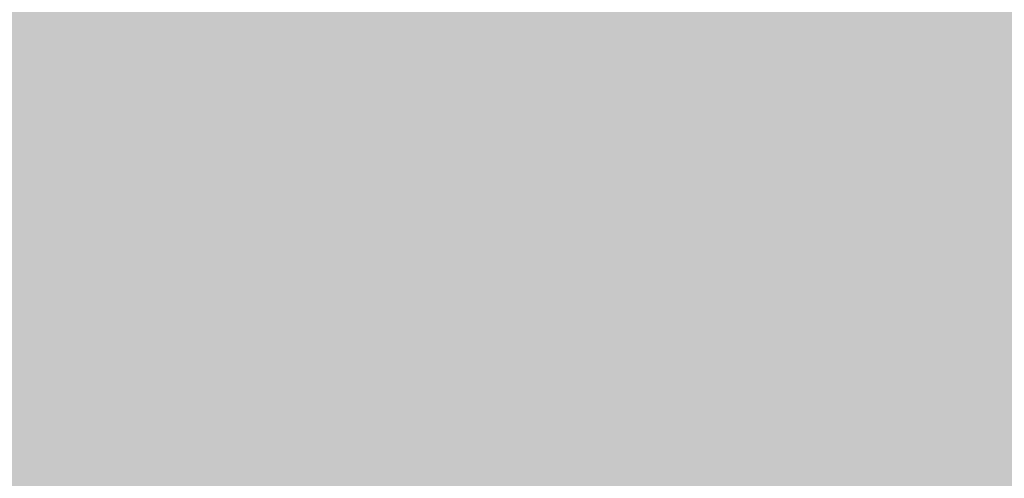
# Model space of a CAD drawing. Units: millimetres. Extents: x 0 to 2267, y 0 to 1823.
# Tile 176 of 256: x 1833.606 to 1838.83, y 1129.713 to 1132.147. Entities that reach past the tile are written whole.
import ezdxf

# ---------------------------------------------------------------- set-up
doc = ezdxf.new("R2010")
doc.units = ezdxf.units.MM
doc.header["$MEASUREMENT"] = 0
doc.layers.add('M-HATC', color=252, linetype='Continuous', lineweight=18)

msp = doc.modelspace()

# ---------------------------------------------------------------- hatches: boundary and pattern name
at = {"layer": 'M-HATC'}
h = msp.add_hatch(color=256, dxfattribs=at)
h.dxf.hatch_style = 1
h.paths.add_polyline_path([(2055.771, 1603.062), (1381.0868, 1603.062), (1381.0868, 1598.062), (2055.771, 1598.062)])
h.paths.add_polyline_path([(2055.771, 1598.062), (1381.0868, 1598.062), (1381.0868, 1593.062), (2055.771, 1593.062)])
h.paths.add_polyline_path([(2051.3074, 1536.7609), (1385.5504, 1536.7609), (1385.5504, 1526.7609), (1387.5504, 1526.7609), (1388.5366, 1525.0528), (1385.3319, 1521.2335), (1385.3319, 1521.2226), (2050.2542, 1522.7491), (2048.3212, 1525.0528), (2049.3074, 1526.7609), (2051.3074, 1526.7609)])
edge = h.paths.add_edge_path()
edge.add_arc((1847.5345, 1379.1492), 135, 222.603061, 222.890851, ccw=False)
edge.add_line((1748.1663, 1287.7656), (1683.0921, 1287.7656))
edge.add_arc((1583.7239, 1379.1492), 135, 317.109149, 317.396939, ccw=False)
edge.add_arc((1678.9686, 1290.6707), 5, 222.8909, 317.1091, ccw=False)
edge.add_arc((1774.2133, 1379.1492), 135, 222.603061, 222.890851, ccw=False)
edge.add_line((1674.8451, 1287.7656), (1609.7709, 1287.7656))
edge.add_arc((1510.4027, 1379.1492), 135, 317.109149, 317.396939, ccw=False)
edge.add_arc((1605.6474, 1290.6707), 5, 222.8909, 317.1091, ccw=False)
edge.add_arc((1700.8921, 1379.1492), 135, 222.603061, 222.890851, ccw=False)
edge.add_line((1601.5239, 1287.7656), (1536.4497, 1287.7656))
edge.add_arc((1437.0815, 1379.1492), 135, 317.109149, 317.396939, ccw=False)
edge.add_arc((1532.3262, 1290.6707), 5, 222.8909, 317.1091, ccw=False)
edge.add_arc((1627.5709, 1379.1492), 135, 222.603061, 222.890851, ccw=False)
edge.add_line((1528.2027, 1287.7656), (1505.9289, 1287.7656))
edge.add_spline(control_points=[(1505.9289, 1287.7656), (1504.2622, 1287.7656), (1504.2622, 1282.7656), (1505.9289, 1282.7656)], knot_values=[0, 0, 0, 0, 5, 5, 5, 5], degree=3, periodic=0)
edge.add_line((1505.9289, 1282.7656), (1930.9289, 1282.7656))
edge.add_spline(control_points=[(1930.9289, 1282.7656), (1932.5956, 1282.7656), (1932.5956, 1287.7656), (1930.9289, 1287.7656)], knot_values=[0, 0, 0, 0, 5, 5, 5, 5], degree=3, periodic=0)
edge.add_line((1930.9289, 1287.7656), (1903.0557, 1287.7656))
edge.add_arc((1803.6875, 1379.1492), 135, 317.109149, 317.396939, ccw=False)
edge.add_arc((1898.9322, 1290.6707), 5, 222.8909, 317.1091, ccw=False)
edge.add_arc((1994.1769, 1379.1492), 135, 222.603061, 222.890851, ccw=False)
edge.add_line((1894.8087, 1287.7656), (1829.7345, 1287.7656))
edge.add_arc((1730.3663, 1379.1492), 135, 317.109149, 317.396939, ccw=False)
edge.add_arc((1825.611, 1290.6707), 5, 222.8909, 317.1091, ccw=False)
edge.add_arc((1920.8557, 1379.1492), 135, 222.603061, 222.890851, ccw=False)
edge.add_line((1821.4875, 1287.7656), (1756.4133, 1287.7656))
edge.add_arc((1657.0451, 1379.1492), 135, 317.109149, 317.396939, ccw=False)
edge.add_arc((1752.2898, 1290.6707), 5, 222.8909, 317.1091, ccw=False)
edge = h.paths.add_edge_path()
edge.add_spline(control_points=[(1843.4289, 1227.2475), (1845.0956, 1227.2475), (1845.0956, 1232.2475), (1843.4289, 1232.2475)], knot_values=[0, 0, 0, 0, 5, 5, 5, 5], degree=3, periodic=0)
edge.add_line((1843.4289, 1232.2475), (1593.4289, 1232.2475))
edge.add_spline(control_points=[(1593.4289, 1232.2475), (1591.7622, 1232.2475), (1591.7622, 1227.2475), (1593.4289, 1227.2475)], knot_values=[0, 0, 0, 0, 5, 5, 5, 5], degree=3, periodic=0)
edge.add_line((1593.4289, 1227.2475), (1843.4289, 1227.2475))
h.paths.add_polyline_path([(1905.9289, 1127.4171), (1530.9289, 1127.4171, 0.414214), (1520.9289, 1117.4171), (1530.9289, 1117.4171), (1915.9289, 1117.4171, 0.414214)])
edge = h.paths.add_edge_path()
edge.add_arc((1397.0858, 1498.4078), 12.7299, 90.78215, 190.87871, ccw=False)
edge.add_line((1396.912, 1511.1365), (1428.0097, 1511.3488))
edge.add_line((1428.0097, 1511.3488), (1433.0097, 1511.3488))
edge.add_line((1433.0097, 1511.3488), (1434.439, 1511.3488))
edge.add_arc((1419.474, 1498.0804), 20, 41.561, 74.08211)
edge.add_line((1424.9592, 1517.3135), (1399.9351, 1517.2561))
edge.add_spline(control_points=[(1399.9307, 1517.2561), (1399.884, 1517.2131), (1399.8328, 1517.1689), (1399.7774, 1517.1236)], knot_values=[11.567499, 11.567499, 11.567499, 11.567499, 11.814249, 11.814249, 11.814249, 11.814249], degree=3, periodic=0)
edge.add_spline(control_points=[(1399.6328, 1517.0099), (1399.5831, 1516.9721), (1399.5307, 1516.9338), (1399.4759, 1516.8947)], knot_values=[11.167718, 11.167718, 11.167718, 11.167718, 11.365188, 11.365188, 11.365188, 11.365188], degree=3, periodic=0)
edge.add_spline(control_points=[(1399.3398, 1516.8001), (1399.1514, 1516.6719), (1398.9384, 1516.5377), (1398.704, 1516.3994)], knot_values=[10.376405, 10.376405, 10.376405, 10.376405, 11.00994, 11.00994, 11.00994, 11.00994], degree=3, periodic=0)
edge.add_spline(control_points=[(1398.6572, 1516.3719), (1398.5789, 1516.326), (1398.4983, 1516.2797), (1398.4155, 1516.2331)], knot_values=[10.125175, 10.125175, 10.125175, 10.125175, 10.334406, 10.334406, 10.334406, 10.334406], degree=3, periodic=0)
edge.add_spline(control_points=[(1398.2642, 1516.1487), (1398.196, 1516.1111), (1398.1263, 1516.0732), (1398.0555, 1516.0351)], knot_values=[9.832246, 9.832246, 9.832246, 9.832246, 9.999658, 9.999658, 9.999658, 9.999658], degree=3, periodic=0)
edge.add_spline(control_points=[(1397.9987, 1516.0048), (1397.7312, 1515.8621), (1397.446, 1515.7171), (1397.1466, 1515.5714)], knot_values=[9.161808, 9.161808, 9.161808, 9.161808, 9.787769, 9.787769, 9.787769, 9.787769], degree=3, periodic=0)
edge.add_spline(control_points=[(1397.1466, 1515.5714), (1396.8418, 1515.423), (1396.5222, 1515.274), (1396.1914, 1515.1262)], knot_values=[8.524455, 8.524455, 8.524455, 8.524455, 9.161808, 9.161808, 9.161808, 9.161808], degree=3, periodic=0)
edge.add_spline(control_points=[(1396.0777, 1515.0756), (1395.9854, 1515.0348), (1395.8922, 1514.994), (1395.7983, 1514.9534)], knot_values=[8.275193, 8.275193, 8.275193, 8.275193, 8.451726, 8.451726, 8.451726, 8.451726], degree=3, periodic=0)
edge.add_spline(control_points=[(1395.6018, 1514.8691), (1395.4997, 1514.8257), (1395.3968, 1514.7824), (1395.2932, 1514.7394)], knot_values=[7.962917, 7.962917, 7.962917, 7.962917, 8.152764, 8.152764, 8.152764, 8.152764], degree=3, periodic=0)
edge.add_spline(control_points=[(1395.2116, 1514.7057), (1394.8278, 1514.5475), (1394.4345, 1514.3929), (1394.0364, 1514.2442)], knot_values=[7.21254, 7.21254, 7.21254, 7.21254, 7.913148, 7.913148, 7.913148, 7.913148], degree=3, periodic=0)
edge.add_spline(control_points=[(1394.0364, 1514.2442), (1393.7076, 1514.1214), (1393.3754, 1514.0027), (1393.0427, 1513.8895)], knot_values=[6.633733, 6.633733, 6.633733, 6.633733, 7.21254, 7.21254, 7.21254, 7.21254], degree=3, periodic=0)
edge.add_spline(control_points=[(1392.8214, 1513.815), (1392.7198, 1513.7812), (1392.6181, 1513.7479), (1392.5166, 1513.7152)], knot_values=[6.328796, 6.328796, 6.328796, 6.328796, 6.505493, 6.505493, 6.505493, 6.505493], degree=3, periodic=0)
edge.add_spline(control_points=[(1392.5166, 1513.7152), (1392.3187, 1513.6515), (1392.1212, 1513.59), (1391.9244, 1513.531)], knot_values=[5.984605, 5.984605, 5.984605, 5.984605, 6.328796, 6.328796, 6.328796, 6.328796], degree=3, periodic=0)
edge.add_spline(control_points=[(1391.7915, 1513.4915), (1391.3122, 1513.3501), (1390.8384, 1513.2239), (1390.3784, 1513.1171)], knot_values=[5.066697, 5.066697, 5.066697, 5.066697, 5.907055, 5.907055, 5.907055, 5.907055], degree=3, periodic=0)
edge.add_spline(control_points=[(1390.3784, 1513.1171), (1390.1797, 1513.071), (1389.9836, 1513.0284), (1389.7907, 1512.9899)], knot_values=[4.70367, 4.70367, 4.70367, 4.70367, 5.066695, 5.066695, 5.066695, 5.066695], degree=3, periodic=0)
edge.add_spline(control_points=[(1389.422, 1512.9204), (1389.2459, 1512.8892), (1389.0729, 1512.8617), (1388.9036, 1512.8381)], knot_values=[4.130571, 4.130571, 4.130571, 4.130571, 4.469816, 4.469816, 4.469816, 4.469816], degree=3, periodic=0)
edge.add_spline(control_points=[(1388.9036, 1512.8381), (1388.591, 1512.7946), (1388.2911, 1512.7644), (1388.0071, 1512.7494)], knot_values=[3.504031, 3.504031, 3.504031, 3.504031, 4.130571, 4.130571, 4.130571, 4.130571], degree=3, periodic=0)
edge.add_spline(control_points=[(1387.9356, 1512.7459), (1387.8538, 1512.7423), (1387.7733, 1512.74), (1387.6944, 1512.739)], knot_values=[3.268866, 3.268866, 3.268866, 3.268866, 3.451164, 3.451164, 3.451164, 3.451164], degree=3, periodic=0)
edge.add_spline(control_points=[(1387.3351, 1512.7443), (1387.2076, 1512.7499), (1387.0847, 1512.7597), (1386.967, 1512.7739)], knot_values=[2.670686, 2.670686, 2.670686, 2.670686, 2.984, 2.984, 2.984, 2.984], degree=3, periodic=0)
edge.add_spline(control_points=[(1386.8327, 1512.7922), (1386.8209, 1512.7941), (1386.8092, 1512.7959), (1386.7975, 1512.7979)], knot_values=[2.516981, 2.516981, 2.516981, 2.516981, 2.549528, 2.549528, 2.549528, 2.549528], degree=3, periodic=0)
edge.add_spline(control_points=[(1386.4526, 1512.8735), (1386.4257, 1512.881), (1386.3993, 1512.889), (1386.3733, 1512.8972)], knot_values=[2.095869, 2.095869, 2.095869, 2.095869, 2.17941, 2.17941, 2.17941, 2.17941], degree=3, periodic=0)
edge.add_spline(control_points=[(1386.0691, 1513.0189), (1386.0634, 1513.0217), (1386.0577, 1513.0246), (1386.052, 1513.0275)], knot_values=[1.72453, 1.72453, 1.72453, 1.72453, 1.745933, 1.745933, 1.745933, 1.745933], degree=3, periodic=0)
edge.add_arc((1399.474, 1498.0804), 20, 131.82432, 180)
edge.add_arc((1630.3336, 1505.5484), 250.9708, 181.705176, 236.427975)
edge.add_arc((1605.3399, 1483.3044), 218.7822, 238.660829, 243.34961)
edge.add_arc((1647.0911, 1510.3592), 262.8986, 183.129836, 237.853442, ccw=False)
h.paths.add_polyline_path([(1406.5369, 1391.9644, 0.149382), (1491.5506, 1296.4418, -0.129517)], flags=17)
edge = h.paths.add_edge_path()
edge.add_arc((2037.3838, 1498.0804), 20, 0, 48.26587)
edge.add_spline(control_points=[(2050.6973, 1513.0052), (2050.6512, 1512.9847), (2050.6034, 1512.9655), (2050.5539, 1512.9477)], knot_values=[1.835652, 1.835652, 1.835652, 1.835652, 2.000781, 2.000781, 2.000781, 2.000781], degree=3, periodic=0)
edge.add_spline(control_points=[(2050.4616, 1512.9166), (2050.479, 1512.9221), (2050.4963, 1512.9277), (2050.5133, 1512.9335)], knot_values=[2.045477, 2.045477, 2.045477, 2.045477, 2.101389, 2.101389, 2.101389, 2.101389], degree=3, periodic=0)
edge.add_spline(control_points=[(2050.129, 1512.8342), (2050.1984, 1512.8473), (2050.2657, 1512.8623), (2050.3308, 1512.8792)], knot_values=[2.237629, 2.237629, 2.237629, 2.237629, 2.435841, 2.435841, 2.435841, 2.435841], degree=3, periodic=0)
edge.add_spline(control_points=[(2050.0946, 1512.8278), (2050.1061, 1512.8299), (2050.1176, 1512.832), (2050.129, 1512.8342)], knot_values=[2.435841, 2.435841, 2.435841, 2.435841, 2.468321, 2.468321, 2.468321, 2.468321], degree=3, periodic=0)
edge.add_spline(control_points=[(2049.7843, 1512.7851), (2049.8552, 1512.7922), (2049.9243, 1512.8008), (2049.9917, 1512.8109)], knot_values=[2.563852, 2.563852, 2.563852, 2.563852, 2.748541, 2.748541, 2.748541, 2.748541], degree=3, periodic=0)
edge.add_spline(control_points=[(2049.4052, 1512.7617), (2049.5364, 1512.7653), (2049.6629, 1512.773), (2049.7843, 1512.7851)], knot_values=[2.748541, 2.748541, 2.748541, 2.748541, 3.064882, 3.064882, 3.064882, 3.064882], degree=3, periodic=0)
edge.add_spline(control_points=[(2049.1698, 1512.7597), (2049.2336, 1512.7591), (2049.2965, 1512.7594), (2049.3584, 1512.7606)], knot_values=[3.102309, 3.102309, 3.102309, 3.102309, 3.2503, 3.2503, 3.2503, 3.2503], degree=3, periodic=0)
edge.add_spline(control_points=[(2048.8573, 1512.7691), (2048.9638, 1512.7638), (2049.068, 1512.7606), (2049.1698, 1512.7597)], knot_values=[3.2503, 3.2503, 3.2503, 3.2503, 3.486069, 3.486069, 3.486069, 3.486069], degree=3, periodic=0)
edge.add_spline(control_points=[(2048.6924, 1512.7789), (2048.3729, 1512.8009), (2048.0345, 1512.8411), (2047.6817, 1512.897)], knot_values=[3.606429, 3.606429, 3.606429, 3.606429, 4.2989, 4.2989, 4.2989, 4.2989], degree=3, periodic=0)
edge.add_spline(control_points=[(2047.6817, 1512.897), (2047.5458, 1512.9185), (2047.4077, 1512.9424), (2047.2678, 1512.9685)], knot_values=[4.2989, 4.2989, 4.2989, 4.2989, 4.565769, 4.565769, 4.565769, 4.565769], degree=3, periodic=0)
edge.add_spline(control_points=[(2047.2678, 1512.9685), (2047.1449, 1512.9914), (2047.0207, 1513.016), (2046.8951, 1513.0422)], knot_values=[4.565769, 4.565769, 4.565769, 4.565769, 4.799971, 4.799971, 4.799971, 4.799971], degree=3, periodic=0)
edge.add_spline(control_points=[(2046.8951, 1513.0422), (2046.5286, 1513.1188), (2046.1513, 1513.209), (2045.7676, 1513.3107)], knot_values=[4.799971, 4.799971, 4.799971, 4.799971, 5.483718, 5.483718, 5.483718, 5.483718], degree=3, periodic=0)
edge.add_spline(control_points=[(2045.7676, 1513.3107), (2045.3724, 1513.4154), (2044.9704, 1513.5322), (2044.5662, 1513.6588)], knot_values=[5.483718, 5.483718, 5.483718, 5.483718, 6.187866, 6.187866, 6.187866, 6.187866], degree=3, periodic=0)
edge.add_spline(control_points=[(2044.5662, 1513.6588), (2044.4149, 1513.7061), (2044.2633, 1513.7549), (2044.1116, 1513.8048)], knot_values=[6.187866, 6.187866, 6.187866, 6.187866, 6.451551, 6.451551, 6.451551, 6.451551], degree=3, periodic=0)
edge.add_spline(control_points=[(2044.1116, 1513.8048), (2043.9967, 1513.8427), (2043.8817, 1513.8813), (2043.7668, 1513.9205)], knot_values=[6.451551, 6.451551, 6.451551, 6.451551, 6.651434, 6.651434, 6.651434, 6.651434], degree=3, periodic=0)
edge.add_spline(control_points=[(2043.7668, 1513.9205), (2043.3716, 1514.0554), (2042.9774, 1514.1979), (2042.5886, 1514.3458)], knot_values=[6.651434, 6.651434, 6.651434, 6.651434, 7.338879, 7.338879, 7.338879, 7.338879], degree=3, periodic=0)
edge.add_spline(control_points=[(2042.5886, 1514.3458), (2042.1643, 1514.5071), (2041.7465, 1514.6749), (2041.3409, 1514.846)], knot_values=[7.338879, 7.338879, 7.338879, 7.338879, 8.089209, 8.089209, 8.089209, 8.089209], degree=3, periodic=0)
edge.add_spline(control_points=[(2041.3409, 1514.846), (2041.1028, 1514.9465), (2040.869, 1515.0481), (2040.6405, 1515.1502)], knot_values=[8.089209, 8.089209, 8.089209, 8.089209, 8.529587, 8.529587, 8.529587, 8.529587], degree=3, periodic=0)
edge.add_spline(control_points=[(2040.51, 1515.2089), (2040.0824, 1515.4022), (2039.6747, 1515.5971), (2039.295, 1515.7894)], knot_values=[8.613818, 8.613818, 8.613818, 8.613818, 9.44571, 9.44571, 9.44571, 9.44571], degree=3, periodic=0)
edge.add_spline(control_points=[(2039.295, 1515.7894), (2039.0618, 1515.9075), (2038.8391, 1516.0246), (2038.6288, 1516.1398)], knot_values=[9.44571, 9.44571, 9.44571, 9.44571, 9.956404, 9.956404, 9.956404, 9.956404], degree=3, periodic=0)
edge.add_spline(control_points=[(2038.6288, 1516.1398), (2038.5187, 1516.2001), (2038.4121, 1516.2598), (2038.309, 1516.3189)], knot_values=[9.956404, 9.956404, 9.956404, 9.956404, 10.223542, 10.223542, 10.223542, 10.223542], degree=3, periodic=0)
edge.add_spline(control_points=[(2038.309, 1516.3189), (2038.2138, 1516.3735), (2038.1216, 1516.4276), (2038.0328, 1516.481)], knot_values=[10.223542, 10.223542, 10.223542, 10.223542, 10.47051, 10.47051, 10.47051, 10.47051], degree=3, periodic=0)
edge.add_spline(control_points=[(2038.0328, 1516.481), (2037.7855, 1516.6296), (2037.5639, 1516.773), (2037.3722, 1516.909)], knot_values=[10.47051, 10.47051, 10.47051, 10.47051, 11.15767, 11.15767, 11.15767, 11.15767], degree=3, periodic=0)
edge.add_spline(control_points=[(2037.3722, 1516.909), (2037.2789, 1516.9752), (2037.1927, 1517.0396), (2037.1142, 1517.102)], knot_values=[11.15767, 11.15767, 11.15767, 11.15767, 11.49227, 11.49227, 11.49227, 11.49227], degree=3, periodic=0)
edge.add_spline(control_points=[(2036.8564, 1517.3259), (2036.9148, 1517.2692), (2036.9814, 1517.2103), (2037.0557, 1517.1492)], knot_values=[11.577341, 11.577341, 11.577341, 11.577341, 11.91035, 11.91035, 11.91035, 11.91035], degree=3, periodic=0)
edge.add_spline(control_points=[(2036.8074, 1517.3748), (2036.823, 1517.3587), (2036.8393, 1517.3424), (2036.8564, 1517.3259)], knot_values=[11.91035, 11.91035, 11.91035, 11.91035, 12.007402, 12.007402, 12.007402, 12.007402], degree=3, periodic=0)
edge.add_spline(control_points=[(2036.7017, 1517.494), (2036.7104, 1517.483), (2036.7196, 1517.4719), (2036.7291, 1517.4606)], knot_values=[12.184155, 12.184155, 12.184155, 12.184155, 12.255409, 12.255409, 12.255409, 12.255409], degree=3, periodic=0)
edge.add_spline(control_points=[(2036.6159, 1517.6205), (2036.62, 1517.613), (2036.6243, 1517.6055), (2036.6289, 1517.5979)], knot_values=[12.487913, 12.487913, 12.487913, 12.487913, 12.541035, 12.541035, 12.541035, 12.541035], degree=3, periodic=0)
edge.add_spline(control_points=[(2036.5635, 1517.786), (2036.5637, 1517.7794), (2036.5642, 1517.7726), (2036.565, 1517.7658)], knot_values=[12.911761, 12.911761, 12.911761, 12.911761, 12.968286, 12.968286, 12.968286, 12.968286], degree=3, periodic=0)
edge.add_spline(control_points=[(2036.6166, 1517.9304), (2036.6125, 1517.9259), (2036.6086, 1517.9212), (2036.6049, 1517.9165)], knot_values=[13.382527, 13.382527, 13.382527, 13.382527, 13.433791, 13.433791, 13.433791, 13.433791], degree=3, periodic=0)
edge.add_spline(control_points=[(2036.749, 1518.017), (2036.7361, 1518.0116), (2036.7239, 1518.006), (2036.7124, 1518.0002)], knot_values=[13.726299, 13.726299, 13.726299, 13.726299, 13.809928, 13.809928, 13.809928, 13.809928], degree=3, periodic=0)
edge.add_spline(control_points=[(2036.8604, 1518.0528), (2036.8386, 1518.0474), (2036.8181, 1518.0416), (2036.7988, 1518.0353)], knot_values=[13.910887, 13.910887, 13.910887, 13.910887, 14.02153, 14.02153, 14.02153, 14.02153], degree=3, periodic=0)
edge.add_line((2036.9639, 1518.0804), (2032.3838, 1518.0804))
edge.add_line((2032.3838, 1518.0804), (2027.3838, 1518.0804))
edge.add_line((2027.3838, 1518.0804), (2022.3838, 1518.0804))
edge.add_line((2022.3838, 1518.0804), (2017.3838, 1518.0804))
edge.add_arc((2017.3838, 1498.0804), 20, 90, 138.439)
edge.add_line((2002.4188, 1511.3488), (2003.8481, 1511.3488))
edge.add_line((2003.8481, 1511.3488), (2008.8481, 1511.3488))
edge.add_line((2008.8481, 1511.3488), (2039.772, 1511.1377))
edge.add_arc((2039.772, 1498.4078), 12.7299, -10.87871, 90, ccw=False)
edge.add_arc((1789.7668, 1510.3592), 262.8986, 302.146558, 356.870164, ccw=False)
edge.add_arc((1831.5179, 1483.3044), 218.7822, 296.65039, 301.339171)
edge.add_arc((1806.5242, 1505.5484), 250.9708, 303.572025, 358.294824)
h.paths.add_polyline_path([(2030.321, 1391.9644, -0.129517), (1945.3072, 1296.4418, 0.149382)], flags=17)
edge = h.paths.add_edge_path()
edge.add_spline(control_points=[(2037.2464, 1518.0821), (2037.2898, 1518.081), (2037.3355, 1518.0804), (2037.3838, 1518.0804)], knot_values=[0.000012, 0.000012, 0.000012, 0.000012, 0.144754, 0.144754, 0.144754, 0.144754], degree=3, periodic=0)
edge.add_line((2037.3357, 1518.0804), (2037.0096, 1518.0804))
edge.add_spline(control_points=[(2037.0096, 1518.0804), (2036.9822, 1518.0768), (2036.956, 1518.0727), (2036.9312, 1518.0681)], knot_values=[14.13465, 14.13465, 14.13465, 14.13465, 14.247197, 14.247197, 14.247197, 14.247197], degree=3, periodic=0)
edge.add_spline(control_points=[(2036.9312, 1518.0681), (2036.9276, 1518.0674), (2036.9241, 1518.0667), (2036.9205, 1518.0661)], knot_values=[14.118315, 14.118315, 14.118315, 14.118315, 14.13465, 14.13465, 14.13465, 14.13465], degree=3, periodic=0)
edge.add_spline(control_points=[(2036.9205, 1518.0661), (2036.9118, 1518.0644), (2036.9032, 1518.0626), (2036.8948, 1518.0608)], knot_values=[14.078086, 14.078086, 14.078086, 14.078086, 14.118315, 14.118315, 14.118315, 14.118315], degree=3, periodic=0)
edge.add_spline(control_points=[(2036.8948, 1518.0608), (2036.883, 1518.0583), (2036.8716, 1518.0556), (2036.8604, 1518.0528)], knot_values=[14.02153, 14.02153, 14.02153, 14.02153, 14.078086, 14.078086, 14.078086, 14.078086], degree=3, periodic=0)
edge.add_spline(control_points=[(2036.8604, 1518.0528), (2036.8386, 1518.0474), (2036.8181, 1518.0416), (2036.7988, 1518.0353)], knot_values=[13.910887, 13.910887, 13.910887, 13.910887, 14.02153, 14.02153, 14.02153, 14.02153], degree=3, periodic=0)
edge.add_spline(control_points=[(2036.7988, 1518.0353), (2036.7981, 1518.035), (2036.7974, 1518.0348), (2036.7967, 1518.0346)], knot_values=[13.906906, 13.906906, 13.906906, 13.906906, 13.910887, 13.910887, 13.910887, 13.910887], degree=3, periodic=0)
edge.add_spline(control_points=[(2036.7967, 1518.0346), (2036.7882, 1518.0318), (2036.7799, 1518.0289), (2036.7719, 1518.0259)], knot_values=[13.857826, 13.857826, 13.857826, 13.857826, 13.906906, 13.906906, 13.906906, 13.906906], degree=3, periodic=0)
edge.add_spline(control_points=[(2036.7719, 1518.0259), (2036.764, 1518.023), (2036.7564, 1518.02), (2036.749, 1518.017)], knot_values=[13.809928, 13.809928, 13.809928, 13.809928, 13.857826, 13.857826, 13.857826, 13.857826], degree=3, periodic=0)
edge.add_spline(control_points=[(2036.749, 1518.017), (2036.7361, 1518.0116), (2036.7239, 1518.006), (2036.7124, 1518.0002)], knot_values=[13.726299, 13.726299, 13.726299, 13.726299, 13.809928, 13.809928, 13.809928, 13.809928], degree=3, periodic=0)
edge.add_spline(control_points=[(2036.7124, 1518.0002), (2036.7121, 1518), (2036.7118, 1517.9999), (2036.7115, 1517.9997)], knot_values=[13.723993, 13.723993, 13.723993, 13.723993, 13.726299, 13.726299, 13.726299, 13.726299], degree=3, periodic=0)
edge.add_spline(control_points=[(2036.7115, 1517.9997), (2036.7063, 1517.9971), (2036.7013, 1517.9944), (2036.6965, 1517.9917)], knot_values=[13.686536, 13.686536, 13.686536, 13.686536, 13.723993, 13.723993, 13.723993, 13.723993], degree=3, periodic=0)
edge.add_spline(control_points=[(2036.6965, 1517.9917), (2036.6919, 1517.9891), (2036.6874, 1517.9865), (2036.6831, 1517.9839)], knot_values=[13.651251, 13.651251, 13.651251, 13.651251, 13.686536, 13.686536, 13.686536, 13.686536], degree=3, periodic=0)
edge.add_spline(control_points=[(2036.6831, 1517.9839), (2036.6764, 1517.9798), (2036.67, 1517.9757), (2036.6639, 1517.9714)], knot_values=[13.596804, 13.596804, 13.596804, 13.596804, 13.651251, 13.651251, 13.651251, 13.651251], degree=3, periodic=0)
edge.add_spline(control_points=[(2036.6639, 1517.9714), (2036.6636, 1517.9712), (2036.6633, 1517.9709), (2036.6629, 1517.9707)], knot_values=[13.593956, 13.593956, 13.593956, 13.593956, 13.596804, 13.596804, 13.596804, 13.596804], degree=3, periodic=0)
edge.add_spline(control_points=[(2036.6629, 1517.9707), (2036.6603, 1517.9689), (2036.6577, 1517.967), (2036.6552, 1517.9651)], knot_values=[13.570322, 13.570322, 13.570322, 13.570322, 13.593956, 13.593956, 13.593956, 13.593956], degree=3, periodic=0)
edge.add_spline(control_points=[(2036.6552, 1517.9651), (2036.6525, 1517.9631), (2036.6499, 1517.9611), (2036.6474, 1517.9591)], knot_values=[13.545477, 13.545477, 13.545477, 13.545477, 13.570322, 13.570322, 13.570322, 13.570322], degree=3, periodic=0)
edge.add_spline(control_points=[(2036.6474, 1517.9591), (2036.6472, 1517.9589), (2036.6471, 1517.9588), (2036.6469, 1517.9587)], knot_values=[13.543931, 13.543931, 13.543931, 13.543931, 13.545477, 13.545477, 13.545477, 13.545477], degree=3, periodic=0)
edge.add_spline(control_points=[(2036.6469, 1517.9587), (2036.6412, 1517.9541), (2036.6358, 1517.9494), (2036.6307, 1517.9447)], knot_values=[13.488237, 13.488237, 13.488237, 13.488237, 13.543931, 13.543931, 13.543931, 13.543931], degree=3, periodic=0)
edge.add_spline(control_points=[(2036.6307, 1517.9447), (2036.6282, 1517.9423), (2036.6257, 1517.9399), (2036.6233, 1517.9374)], knot_values=[13.460307, 13.460307, 13.460307, 13.460307, 13.488237, 13.488237, 13.488237, 13.488237], degree=3, periodic=0)
edge.add_spline(control_points=[(2036.6233, 1517.9374), (2036.6215, 1517.9356), (2036.6198, 1517.9338), (2036.6181, 1517.932)], knot_values=[13.439712, 13.439712, 13.439712, 13.439712, 13.460307, 13.460307, 13.460307, 13.460307], degree=3, periodic=0)
edge.add_spline(control_points=[(2036.6181, 1517.932), (2036.6176, 1517.9315), (2036.6171, 1517.9309), (2036.6166, 1517.9304)], knot_values=[13.433791, 13.433791, 13.433791, 13.433791, 13.439712, 13.439712, 13.439712, 13.439712], degree=3, periodic=0)
edge.add_spline(control_points=[(2036.6166, 1517.9304), (2036.6125, 1517.9259), (2036.6086, 1517.9212), (2036.6049, 1517.9165)], knot_values=[13.382527, 13.382527, 13.382527, 13.382527, 13.433791, 13.433791, 13.433791, 13.433791], degree=3, periodic=0)
edge.add_spline(control_points=[(2036.6049, 1517.9165), (2036.6026, 1517.9135), (2036.6004, 1517.9104), (2036.5982, 1517.9074)], knot_values=[13.350017, 13.350017, 13.350017, 13.350017, 13.382527, 13.382527, 13.382527, 13.382527], degree=3, periodic=0)
edge.add_spline(control_points=[(2036.5982, 1517.9074), (2036.5972, 1517.9059), (2036.5962, 1517.9043), (2036.5952, 1517.9028)], knot_values=[13.333922, 13.333922, 13.333922, 13.333922, 13.350017, 13.350017, 13.350017, 13.350017], degree=3, periodic=0)
edge.add_spline(control_points=[(2036.5952, 1517.9028), (2036.5945, 1517.9018), (2036.5939, 1517.9009), (2036.5933, 1517.8999)], knot_values=[13.323828, 13.323828, 13.323828, 13.323828, 13.333922, 13.333922, 13.333922, 13.333922], degree=3, periodic=0)
edge.add_spline(control_points=[(2036.5933, 1517.8999), (2036.5905, 1517.8955), (2036.5879, 1517.8909), (2036.5855, 1517.8864)], knot_values=[13.277545, 13.277545, 13.277545, 13.277545, 13.323828, 13.323828, 13.323828, 13.323828], degree=3, periodic=0)
edge.add_spline(control_points=[(2036.5855, 1517.8864), (2036.5836, 1517.8827), (2036.5817, 1517.8789), (2036.5801, 1517.8751)], knot_values=[13.240119, 13.240119, 13.240119, 13.240119, 13.277545, 13.277545, 13.277545, 13.277545], degree=3, periodic=0)
edge.add_spline(control_points=[(2036.5801, 1517.8751), (2036.5795, 1517.8739), (2036.579, 1517.8727), (2036.5785, 1517.8715)], knot_values=[13.228211, 13.228211, 13.228211, 13.228211, 13.240119, 13.240119, 13.240119, 13.240119], degree=3, periodic=0)
edge.add_spline(control_points=[(2036.5785, 1517.8715), (2036.578, 1517.8702), (2036.5774, 1517.869), (2036.5769, 1517.8677)], knot_values=[13.215717, 13.215717, 13.215717, 13.215717, 13.228211, 13.228211, 13.228211, 13.228211], degree=3, periodic=0)
edge.add_spline(control_points=[(2036.5769, 1517.8677), (2036.5755, 1517.864), (2036.5741, 1517.8603), (2036.5729, 1517.8565)], knot_values=[13.179847, 13.179847, 13.179847, 13.179847, 13.215717, 13.215717, 13.215717, 13.215717], degree=3, periodic=0)
edge.add_spline(control_points=[(2036.5729, 1517.8565), (2036.5713, 1517.8515), (2036.5699, 1517.8464), (2036.5687, 1517.8413)], knot_values=[13.132017, 13.132017, 13.132017, 13.132017, 13.179847, 13.179847, 13.179847, 13.179847], degree=3, periodic=0)
edge.add_spline(control_points=[(2036.5687, 1517.8413), (2036.5684, 1517.8402), (2036.5682, 1517.8392), (2036.568, 1517.8382)], knot_values=[13.122482, 13.122482, 13.122482, 13.122482, 13.132017, 13.132017, 13.132017, 13.132017], degree=3, periodic=0)
edge.add_spline(control_points=[(2036.568, 1517.8382), (2036.5676, 1517.8363), (2036.5672, 1517.8345), (2036.5669, 1517.8327)], knot_values=[13.105592, 13.105592, 13.105592, 13.105592, 13.122482, 13.122482, 13.122482, 13.122482], degree=3, periodic=0)
edge.add_spline(control_points=[(2036.5669, 1517.8327), (2036.5662, 1517.8292), (2036.5657, 1517.8257), (2036.5652, 1517.8222)], knot_values=[13.074063, 13.074063, 13.074063, 13.074063, 13.105592, 13.105592, 13.105592, 13.105592], degree=3, periodic=0)
edge.add_spline(control_points=[(2036.5652, 1517.8222), (2036.5652, 1517.8222), (2036.5652, 1517.8222), (2036.5652, 1517.8222)], knot_values=[13.074043, 13.074043, 13.074043, 13.074043, 13.074063, 13.074063, 13.074063, 13.074063], degree=3, periodic=0)
edge.add_spline(control_points=[(2036.5652, 1517.8222), (2036.5644, 1517.8164), (2036.5639, 1517.8106), (2036.5636, 1517.8046)], knot_values=[13.021884, 13.021884, 13.021884, 13.021884, 13.074043, 13.074043, 13.074043, 13.074043], degree=3, periodic=0)
edge.add_spline(control_points=[(2036.5636, 1517.8046), (2036.5636, 1517.804), (2036.5636, 1517.8034), (2036.5635, 1517.8028)], knot_values=[13.01674, 13.01674, 13.01674, 13.01674, 13.021884, 13.021884, 13.021884, 13.021884], degree=3, periodic=0)
edge.add_spline(control_points=[(2036.5635, 1517.8028), (2036.5634, 1517.8005), (2036.5634, 1517.7982), (2036.5634, 1517.7958)], knot_values=[12.996438, 12.996438, 12.996438, 12.996438, 13.01674, 13.01674, 13.01674, 13.01674], degree=3, periodic=0)
edge.add_spline(control_points=[(2036.5634, 1517.7958), (2036.5633, 1517.7926), (2036.5634, 1517.7893), (2036.5635, 1517.786)], knot_values=[12.968286, 12.968286, 12.968286, 12.968286, 12.996438, 12.996438, 12.996438, 12.996438], degree=3, periodic=0)
edge.add_spline(control_points=[(2036.5635, 1517.786), (2036.5637, 1517.7794), (2036.5642, 1517.7726), (2036.565, 1517.7658)], knot_values=[12.911761, 12.911761, 12.911761, 12.911761, 12.968286, 12.968286, 12.968286, 12.968286], degree=3, periodic=0)
edge.add_spline(control_points=[(2036.565, 1517.7658), (2036.565, 1517.7657), (2036.565, 1517.7656), (2036.565, 1517.7656)], knot_values=[12.911017, 12.911017, 12.911017, 12.911017, 12.911761, 12.911761, 12.911761, 12.911761], degree=3, periodic=0)
edge.add_spline(control_points=[(2036.565, 1517.7656), (2036.5654, 1517.7625), (2036.5658, 1517.7593), (2036.5663, 1517.7562)], knot_values=[12.88528, 12.88528, 12.88528, 12.88528, 12.911017, 12.911017, 12.911017, 12.911017], degree=3, periodic=0)
edge.add_spline(control_points=[(2036.5663, 1517.7562), (2036.5667, 1517.7534), (2036.5672, 1517.7506), (2036.5677, 1517.7478)], knot_values=[12.862519, 12.862519, 12.862519, 12.862519, 12.88528, 12.88528, 12.88528, 12.88528], degree=3, periodic=0)
edge.add_spline(control_points=[(2036.5677, 1517.7478), (2036.5678, 1517.7474), (2036.5679, 1517.7469), (2036.568, 1517.7465)], knot_values=[12.858885, 12.858885, 12.858885, 12.858885, 12.862519, 12.862519, 12.862519, 12.862519], degree=3, periodic=0)
edge.add_spline(control_points=[(2036.568, 1517.7465), (2036.5692, 1517.7399), (2036.5707, 1517.7332), (2036.5724, 1517.7264)], knot_values=[12.8053, 12.8053, 12.8053, 12.8053, 12.858885, 12.858885, 12.858885, 12.858885], degree=3, periodic=0)
edge.add_spline(control_points=[(2036.5724, 1517.7264), (2036.5734, 1517.7226), (2036.5745, 1517.7187), (2036.5756, 1517.7149)], knot_values=[12.775176, 12.775176, 12.775176, 12.775176, 12.8053, 12.8053, 12.8053, 12.8053], degree=3, periodic=0)
edge.add_spline(control_points=[(2036.5756, 1517.7149), (2036.5763, 1517.7125), (2036.577, 1517.7102), (2036.5778, 1517.7078)], knot_values=[12.756759, 12.756759, 12.756759, 12.756759, 12.775176, 12.775176, 12.775176, 12.775176], degree=3, periodic=0)
edge.add_spline(control_points=[(2036.5778, 1517.7078), (2036.5781, 1517.7067), (2036.5784, 1517.7057), (2036.5787, 1517.7047)], knot_values=[12.748742, 12.748742, 12.748742, 12.748742, 12.756759, 12.756759, 12.756759, 12.756759], degree=3, periodic=0)
edge.add_spline(control_points=[(2036.5787, 1517.7047), (2036.5808, 1517.6983), (2036.5831, 1517.6919), (2036.5856, 1517.6854)], knot_values=[12.69959, 12.69959, 12.69959, 12.69959, 12.748742, 12.748742, 12.748742, 12.748742], degree=3, periodic=0)
edge.add_spline(control_points=[(2036.5856, 1517.6854), (2036.5876, 1517.68), (2036.5898, 1517.6746), (2036.5921, 1517.6692)], knot_values=[12.659038, 12.659038, 12.659038, 12.659038, 12.69959, 12.69959, 12.69959, 12.69959], degree=3, periodic=0)
edge.add_spline(control_points=[(2036.5921, 1517.6692), (2036.594, 1517.6648), (2036.5959, 1517.6605), (2036.5979, 1517.6561)], knot_values=[12.626806, 12.626806, 12.626806, 12.626806, 12.659038, 12.659038, 12.659038, 12.659038], degree=3, periodic=0)
edge.add_spline(control_points=[(2036.5979, 1517.6561), (2036.5984, 1517.6551), (2036.5989, 1517.6541), (2036.5993, 1517.6531)], knot_values=[12.619394, 12.619394, 12.619394, 12.619394, 12.626806, 12.626806, 12.626806, 12.626806], degree=3, periodic=0)
edge.add_spline(control_points=[(2036.5993, 1517.6531), (2036.6043, 1517.6424), (2036.6099, 1517.6315), (2036.6159, 1517.6205)], knot_values=[12.541039, 12.541039, 12.541039, 12.541039, 12.619394, 12.619394, 12.619394, 12.619394], degree=3, periodic=0)
edge.add_spline(control_points=[(2036.6159, 1517.6205), (2036.6159, 1517.6205), (2036.6159, 1517.6205), (2036.6159, 1517.6205)], knot_values=[12.541035, 12.541035, 12.541035, 12.541035, 12.541039, 12.541039, 12.541039, 12.541039], degree=3, periodic=0)
edge.add_spline(control_points=[(2036.6159, 1517.6205), (2036.62, 1517.613), (2036.6243, 1517.6055), (2036.6289, 1517.5979)], knot_values=[12.487913, 12.487913, 12.487913, 12.487913, 12.541035, 12.541035, 12.541035, 12.541035], degree=3, periodic=0)
edge.add_spline(control_points=[(2036.6289, 1517.5979), (2036.6326, 1517.5916), (2036.6365, 1517.5853), (2036.6406, 1517.5789)], knot_values=[12.443982, 12.443982, 12.443982, 12.443982, 12.487913, 12.487913, 12.487913, 12.487913], degree=3, periodic=0)
edge.add_spline(control_points=[(2036.6406, 1517.5789), (2036.6414, 1517.5776), (2036.6423, 1517.5763), (2036.6431, 1517.5749)], knot_values=[12.434996, 12.434996, 12.434996, 12.434996, 12.443982, 12.443982, 12.443982, 12.443982], degree=3, periodic=0)
edge.add_spline(control_points=[(2036.6431, 1517.5749), (2036.6531, 1517.5596), (2036.6639, 1517.5439), (2036.6756, 1517.528)], knot_values=[12.329647, 12.329647, 12.329647, 12.329647, 12.434996, 12.434996, 12.434996, 12.434996], degree=3, periodic=0)
edge.add_spline(control_points=[(2036.6756, 1517.528), (2036.6839, 1517.5168), (2036.6925, 1517.5055), (2036.7017, 1517.494)], knot_values=[12.255409, 12.255409, 12.255409, 12.255409, 12.329647, 12.329647, 12.329647, 12.329647], degree=3, periodic=0)
edge.add_spline(control_points=[(2036.7017, 1517.494), (2036.7104, 1517.483), (2036.7196, 1517.4719), (2036.7291, 1517.4606)], knot_values=[12.184155, 12.184155, 12.184155, 12.184155, 12.255409, 12.255409, 12.255409, 12.255409], degree=3, periodic=0)
edge.add_spline(control_points=[(2036.7291, 1517.4606), (2036.7436, 1517.4435), (2036.759, 1517.4262), (2036.7753, 1517.4085)], knot_values=[12.075961, 12.075961, 12.075961, 12.075961, 12.184155, 12.184155, 12.184155, 12.184155], degree=3, periodic=0)
edge.add_spline(control_points=[(2036.7753, 1517.4085), (2036.7763, 1517.4075), (2036.7773, 1517.4064), (2036.7783, 1517.4054)], knot_values=[12.069502, 12.069502, 12.069502, 12.069502, 12.075961, 12.075961, 12.075961, 12.075961], degree=3, periodic=0)
edge.add_spline(control_points=[(2036.7783, 1517.4054), (2036.7877, 1517.3953), (2036.7974, 1517.385), (2036.8074, 1517.3748)], knot_values=[12.007402, 12.007402, 12.007402, 12.007402, 12.069502, 12.069502, 12.069502, 12.069502], degree=3, periodic=0)
edge.add_spline(control_points=[(2036.8074, 1517.3748), (2036.823, 1517.3587), (2036.8393, 1517.3424), (2036.8564, 1517.3259)], knot_values=[11.91035, 11.91035, 11.91035, 11.91035, 12.007402, 12.007402, 12.007402, 12.007402], degree=3, periodic=0)
edge.add_spline(control_points=[(2036.8564, 1517.3259), (2036.9148, 1517.2692), (2036.9814, 1517.2103), (2037.0557, 1517.1492)], knot_values=[11.577341, 11.577341, 11.577341, 11.577341, 11.91035, 11.91035, 11.91035, 11.91035], degree=3, periodic=0)
edge.add_spline(control_points=[(2037.0557, 1517.1492), (2037.0747, 1517.1336), (2037.0942, 1517.1179), (2037.1142, 1517.102)], knot_values=[11.49227, 11.49227, 11.49227, 11.49227, 11.577341, 11.577341, 11.577341, 11.577341], degree=3, periodic=0)
edge.add_spline(control_points=[(2037.1142, 1517.102), (2037.1927, 1517.0396), (2037.2789, 1516.9752), (2037.3722, 1516.909)], knot_values=[11.15767, 11.15767, 11.15767, 11.15767, 11.49227, 11.49227, 11.49227, 11.49227], degree=3, periodic=0)
edge.add_spline(control_points=[(2037.3722, 1516.909), (2037.5639, 1516.773), (2037.7855, 1516.6296), (2038.0328, 1516.481)], knot_values=[10.47051, 10.47051, 10.47051, 10.47051, 11.15767, 11.15767, 11.15767, 11.15767], degree=3, periodic=0)
edge.add_spline(control_points=[(2038.0328, 1516.481), (2038.1216, 1516.4276), (2038.2138, 1516.3735), (2038.309, 1516.3189)], knot_values=[10.223542, 10.223542, 10.223542, 10.223542, 10.47051, 10.47051, 10.47051, 10.47051], degree=3, periodic=0)
edge.add_spline(control_points=[(2038.309, 1516.3189), (2038.4121, 1516.2598), (2038.5187, 1516.2001), (2038.6288, 1516.1398)], knot_values=[9.956404, 9.956404, 9.956404, 9.956404, 10.223542, 10.223542, 10.223542, 10.223542], degree=3, periodic=0)
edge.add_spline(control_points=[(2038.6288, 1516.1398), (2038.8391, 1516.0246), (2039.0618, 1515.9075), (2039.295, 1515.7894)], knot_values=[9.44571, 9.44571, 9.44571, 9.44571, 9.956404, 9.956404, 9.956404, 9.956404], degree=3, periodic=0)
edge.add_spline(control_points=[(2039.295, 1515.7894), (2039.6747, 1515.5971), (2040.0824, 1515.4022), (2040.51, 1515.2089)], knot_values=[8.613818, 8.613818, 8.613818, 8.613818, 9.44571, 9.44571, 9.44571, 9.44571], degree=3, periodic=0)
edge.add_spline(control_points=[(2040.51, 1515.2089), (2040.5533, 1515.1893), (2040.5968, 1515.1697), (2040.6405, 1515.1502)], knot_values=[8.529587, 8.529587, 8.529587, 8.529587, 8.613818, 8.613818, 8.613818, 8.613818], degree=3, periodic=0)
edge.add_spline(control_points=[(2040.6405, 1515.1502), (2040.869, 1515.0481), (2041.1028, 1514.9465), (2041.3409, 1514.846)], knot_values=[8.089209, 8.089209, 8.089209, 8.089209, 8.529587, 8.529587, 8.529587, 8.529587], degree=3, periodic=0)
edge.add_spline(control_points=[(2041.3409, 1514.846), (2041.7465, 1514.6749), (2042.1643, 1514.5071), (2042.5886, 1514.3458)], knot_values=[7.338879, 7.338879, 7.338879, 7.338879, 8.089209, 8.089209, 8.089209, 8.089209], degree=3, periodic=0)
edge.add_spline(control_points=[(2042.5886, 1514.3458), (2042.9774, 1514.1979), (2043.3716, 1514.0554), (2043.7668, 1513.9205)], knot_values=[6.651434, 6.651434, 6.651434, 6.651434, 7.338879, 7.338879, 7.338879, 7.338879], degree=3, periodic=0)
edge.add_spline(control_points=[(2043.7668, 1513.9205), (2043.8817, 1513.8813), (2043.9967, 1513.8427), (2044.1116, 1513.8048)], knot_values=[6.451551, 6.451551, 6.451551, 6.451551, 6.651434, 6.651434, 6.651434, 6.651434], degree=3, periodic=0)
edge.add_spline(control_points=[(2044.1116, 1513.8048), (2044.2633, 1513.7549), (2044.4149, 1513.7061), (2044.5662, 1513.6588)], knot_values=[6.187866, 6.187866, 6.187866, 6.187866, 6.451551, 6.451551, 6.451551, 6.451551], degree=3, periodic=0)
edge.add_spline(control_points=[(2044.5662, 1513.6588), (2044.9704, 1513.5322), (2045.3724, 1513.4154), (2045.7676, 1513.3107)], knot_values=[5.483718, 5.483718, 5.483718, 5.483718, 6.187866, 6.187866, 6.187866, 6.187866], degree=3, periodic=0)
edge.add_spline(control_points=[(2045.7676, 1513.3107), (2046.1513, 1513.209), (2046.5286, 1513.1188), (2046.8951, 1513.0422)], knot_values=[4.799971, 4.799971, 4.799971, 4.799971, 5.483718, 5.483718, 5.483718, 5.483718], degree=3, periodic=0)
edge.add_spline(control_points=[(2046.8951, 1513.0422), (2047.0207, 1513.016), (2047.1449, 1512.9914), (2047.2678, 1512.9685)], knot_values=[4.565769, 4.565769, 4.565769, 4.565769, 4.799971, 4.799971, 4.799971, 4.799971], degree=3, periodic=0)
edge.add_spline(control_points=[(2047.2678, 1512.9685), (2047.4077, 1512.9424), (2047.5458, 1512.9185), (2047.6817, 1512.897)], knot_values=[4.2989, 4.2989, 4.2989, 4.2989, 4.565769, 4.565769, 4.565769, 4.565769], degree=3, periodic=0)
edge.add_spline(control_points=[(2047.6817, 1512.897), (2048.0345, 1512.8411), (2048.3729, 1512.8009), (2048.6924, 1512.7789)], knot_values=[3.606429, 3.606429, 3.606429, 3.606429, 4.2989, 4.2989, 4.2989, 4.2989], degree=3, periodic=0)
edge.add_spline(control_points=[(2048.6924, 1512.7789), (2048.7479, 1512.7751), (2048.8029, 1512.7718), (2048.8573, 1512.7691)], knot_values=[3.486069, 3.486069, 3.486069, 3.486069, 3.606429, 3.606429, 3.606429, 3.606429], degree=3, periodic=0)
edge.add_spline(control_points=[(2048.8573, 1512.7691), (2048.9638, 1512.7638), (2049.068, 1512.7606), (2049.1698, 1512.7597)], knot_values=[3.2503, 3.2503, 3.2503, 3.2503, 3.486069, 3.486069, 3.486069, 3.486069], degree=3, periodic=0)
edge.add_spline(control_points=[(2049.1698, 1512.7597), (2049.2336, 1512.7591), (2049.2965, 1512.7594), (2049.3584, 1512.7606)], knot_values=[3.102309, 3.102309, 3.102309, 3.102309, 3.2503, 3.2503, 3.2503, 3.2503], degree=3, periodic=0)
edge.add_spline(control_points=[(2049.3584, 1512.7606), (2049.3741, 1512.7609), (2049.3897, 1512.7613), (2049.4052, 1512.7617)], knot_values=[3.064882, 3.064882, 3.064882, 3.064882, 3.102309, 3.102309, 3.102309, 3.102309], degree=3, periodic=0)
edge.add_spline(control_points=[(2049.4052, 1512.7617), (2049.5364, 1512.7653), (2049.6629, 1512.773), (2049.7843, 1512.7851)], knot_values=[2.748541, 2.748541, 2.748541, 2.748541, 3.064882, 3.064882, 3.064882, 3.064882], degree=3, periodic=0)
edge.add_spline(control_points=[(2049.7843, 1512.7851), (2049.8552, 1512.7922), (2049.9243, 1512.8008), (2049.9917, 1512.8109)], knot_values=[2.563852, 2.563852, 2.563852, 2.563852, 2.748541, 2.748541, 2.748541, 2.748541], degree=3, periodic=0)
edge.add_spline(control_points=[(2049.9917, 1512.8109), (2050.0265, 1512.8161), (2050.0608, 1512.8218), (2050.0946, 1512.8278)], knot_values=[2.468321, 2.468321, 2.468321, 2.468321, 2.563852, 2.563852, 2.563852, 2.563852], degree=3, periodic=0)
edge.add_spline(control_points=[(2050.0946, 1512.8278), (2050.1061, 1512.8299), (2050.1176, 1512.832), (2050.129, 1512.8342)], knot_values=[2.435841, 2.435841, 2.435841, 2.435841, 2.468321, 2.468321, 2.468321, 2.468321], degree=3, periodic=0)
edge.add_spline(control_points=[(2050.129, 1512.8342), (2050.1984, 1512.8473), (2050.2657, 1512.8623), (2050.3308, 1512.8792)], knot_values=[2.237629, 2.237629, 2.237629, 2.237629, 2.435841, 2.435841, 2.435841, 2.435841], degree=3, periodic=0)
edge.add_spline(control_points=[(2050.3308, 1512.8792), (2050.3754, 1512.8908), (2050.4191, 1512.9032), (2050.4616, 1512.9166)], knot_values=[2.101389, 2.101389, 2.101389, 2.101389, 2.237629, 2.237629, 2.237629, 2.237629], degree=3, periodic=0)
edge.add_spline(control_points=[(2050.4616, 1512.9166), (2050.479, 1512.9221), (2050.4963, 1512.9277), (2050.5133, 1512.9335)], knot_values=[2.045477, 2.045477, 2.045477, 2.045477, 2.101389, 2.101389, 2.101389, 2.101389], degree=3, periodic=0)
edge.add_spline(control_points=[(2050.5133, 1512.9335), (2050.527, 1512.9382), (2050.5405, 1512.9429), (2050.5539, 1512.9477)], knot_values=[2.000781, 2.000781, 2.000781, 2.000781, 2.045477, 2.045477, 2.045477, 2.045477], degree=3, periodic=0)
edge.add_spline(control_points=[(2050.5539, 1512.9477), (2050.6034, 1512.9655), (2050.6512, 1512.9847), (2050.6973, 1513.0052)], knot_values=[1.835652, 1.835652, 1.835652, 1.835652, 2.000781, 2.000781, 2.000781, 2.000781], degree=3, periodic=0)
edge.add_arc((2037.3838, 1498.0804), 20, 48.26587, 90.12993)
edge = h.paths.add_edge_path(flags=16)
edge.add_spline(control_points=[(1386.1389, 1512.9859), (1388.92, 1511.7395), (1398.0387, 1515.5187), (1399.9307, 1517.2561)], knot_values=[1.831046, 1.831046, 1.831046, 1.831046, 11.814249, 11.814249, 11.814249, 11.814249], degree=3, periodic=0)
edge.add_line((1399.9307, 1517.2561), (1393.7435, 1517.2419))
edge.add_arc((1399.474, 1498.0804), 20, 106.6501, 131.8173)
h = msp.add_hatch(color=256, dxfattribs=at)
h.dxf.hatch_style = 1
h.paths.add_polyline_path([(2042.8886, 1580.1796), (2055.771, 1593.062), (1381.0868, 1593.062), (1393.9692, 1580.1796), (1374.086, 1560.2964), (2062.7718, 1560.2964)])
h.paths.add_polyline_path([(1843.4289, 1201.3297), (1843.4289, 1227.2475), (1593.4289, 1227.2475), (1593.4289, 1201.3297, -0.228274), (1574.5989, 1162.2346), (1530.9289, 1127.4171), (1905.9289, 1127.4171), (1862.2589, 1162.2346, -0.228274)])

doc.saveas('drawing.dxf')
